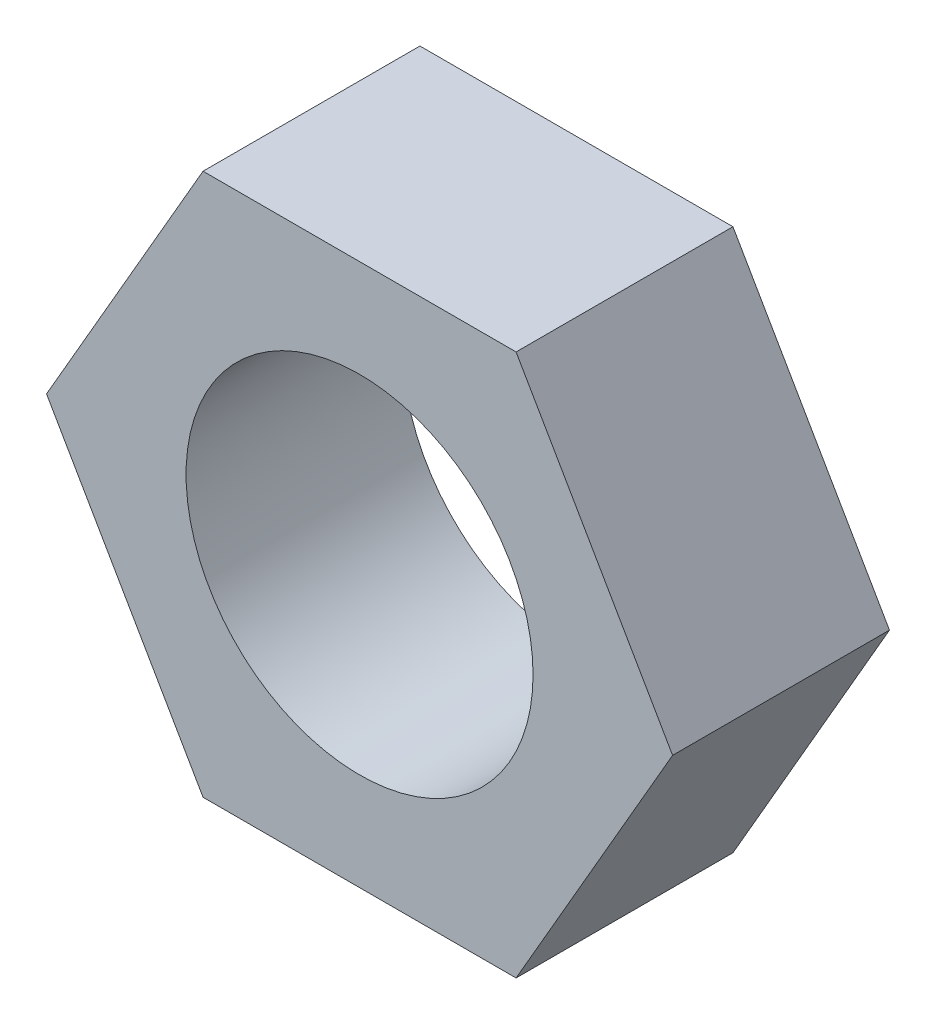
ISO-10303-21;
HEADER;
FILE_DESCRIPTION(('STEP AP214'),'2;1');
FILE_NAME('part.step','',(''),(''),'','','');
FILE_SCHEMA(('AUTOMOTIVE_DESIGN { 1 0 10303 214 1 1 1 1 }'));
ENDSEC;
DATA;
#1=APPLICATION_CONTEXT('core data for automotive mechanical design processes');
#2=APPLICATION_PROTOCOL_DEFINITION('international standard','automotive_design',2000,#1);
#3=PRODUCT_CONTEXT('',#1,'mechanical');
#4=PRODUCT('Part','Part','',(#3));
#5=PRODUCT_RELATED_PRODUCT_CATEGORY('part','',(#4));
#6=PRODUCT_DEFINITION_FORMATION('','',#4);
#7=PRODUCT_DEFINITION_CONTEXT('part definition',#1,'design');
#8=PRODUCT_DEFINITION('design','',#6,#7);
#9=PRODUCT_DEFINITION_SHAPE('','',#8);
#10=(LENGTH_UNIT() NAMED_UNIT(*) SI_UNIT(.MILLI.,.METRE.));
#11=(NAMED_UNIT(*) PLANE_ANGLE_UNIT() SI_UNIT($,.RADIAN.));
#12=(NAMED_UNIT(*) SI_UNIT($,.STERADIAN.) SOLID_ANGLE_UNIT());
#13=UNCERTAINTY_MEASURE_WITH_UNIT(LENGTH_MEASURE(1.E-05),#10,'distance_accuracy_value','');
#14=(GEOMETRIC_REPRESENTATION_CONTEXT(3) GLOBAL_UNCERTAINTY_ASSIGNED_CONTEXT((#13)) GLOBAL_UNIT_ASSIGNED_CONTEXT((#10,
#11,#12)) REPRESENTATION_CONTEXT('',''));
#15=CARTESIAN_POINT('',(0.,0.,0.));
#16=DIRECTION('',(0.,0.,1.));
#17=DIRECTION('',(1.,0.,0.));
#18=AXIS2_PLACEMENT_3D('',#15,#16,#17);
#19=CARTESIAN_POINT('',(7.21687836487047,-12.4999999999999,10.));
#20=DIRECTION('',(-0.866025403784442,0.499999999999995,0.));
#21=DIRECTION('',(-0.499999999999995,-0.866025403784442,0.));
#22=AXIS2_PLACEMENT_3D('',#19,#20,#21);
#23=PLANE('',#22);
#24=DIRECTION('',(0.499999999999995,0.866025403784442,0.));
#25=VECTOR('',#24,1.);
#26=CARTESIAN_POINT('',(7.21687836487047,-12.4999999999999,0.));
#27=LINE('',#26,#25);
#28=CARTESIAN_POINT('',(7.21687836487047,-12.4999999999999,0.));
#29=VERTEX_POINT('',#28);
#30=CARTESIAN_POINT('',(14.4337567297407,0.,0.));
#31=VERTEX_POINT('',#30);
#32=EDGE_CURVE('E122',#29,#31,#27,.T.);
#33=ORIENTED_EDGE('',*,*,#32,.T.);
#34=DIRECTION('',(0.,0.,-1.));
#35=VECTOR('',#34,1.);
#36=CARTESIAN_POINT('',(14.4337567297407,0.,10.));
#37=LINE('',#36,#35);
#38=CARTESIAN_POINT('',(14.4337567297407,0.,10.));
#39=VERTEX_POINT('',#38);
#40=EDGE_CURVE('E11',#39,#31,#37,.T.);
#41=ORIENTED_EDGE('',*,*,#40,.F.);
#42=DIRECTION('',(0.499999999999995,0.866025403784442,0.));
#43=VECTOR('',#42,1.);
#44=CARTESIAN_POINT('',(7.21687836487047,-12.4999999999999,10.));
#45=LINE('',#44,#43);
#46=CARTESIAN_POINT('',(7.21687836487047,-12.4999999999999,10.));
#47=VERTEX_POINT('',#46);
#48=EDGE_CURVE('E133',#47,#39,#45,.T.);
#49=ORIENTED_EDGE('',*,*,#48,.F.);
#50=DIRECTION('',(0.,0.,-1.));
#51=VECTOR('',#50,1.);
#52=CARTESIAN_POINT('',(7.21687836487047,-12.4999999999999,10.));
#53=LINE('',#52,#51);
#54=EDGE_CURVE('E118',#47,#29,#53,.T.);
#55=ORIENTED_EDGE('',*,*,#54,.T.);
#56=EDGE_LOOP('',(#33,#41,#49,#55));
#57=FACE_BOUND('',#56,.T.);
#58=ADVANCED_FACE('F39',(#57),#23,.F.);
#59=CARTESIAN_POINT('',(14.4337567297407,0.,10.));
#60=DIRECTION('',(-0.866025403784438,-0.500000000000001,0.));
#61=DIRECTION('',(0.500000000000001,-0.866025403784438,0.));
#62=AXIS2_PLACEMENT_3D('',#59,#60,#61);
#63=PLANE('',#62);
#64=DIRECTION('',(-0.500000000000001,0.866025403784438,0.));
#65=VECTOR('',#64,1.);
#66=CARTESIAN_POINT('',(14.4337567297407,0.,0.));
#67=LINE('',#66,#65);
#68=CARTESIAN_POINT('',(7.2168783648703,12.5,0.));
#69=VERTEX_POINT('',#68);
#70=EDGE_CURVE('E127',#31,#69,#67,.T.);
#71=ORIENTED_EDGE('',*,*,#70,.T.);
#72=DIRECTION('',(0.,0.,-1.));
#73=VECTOR('',#72,1.);
#74=CARTESIAN_POINT('',(7.2168783648703,12.5,10.));
#75=LINE('',#74,#73);
#76=CARTESIAN_POINT('',(7.2168783648703,12.5,10.));
#77=VERTEX_POINT('',#76);
#78=EDGE_CURVE('E50',#77,#69,#75,.T.);
#79=ORIENTED_EDGE('',*,*,#78,.F.);
#80=DIRECTION('',(-0.500000000000001,0.866025403784438,0.));
#81=VECTOR('',#80,1.);
#82=CARTESIAN_POINT('',(14.4337567297407,0.,10.));
#83=LINE('',#82,#81);
#84=EDGE_CURVE('E95',#39,#77,#83,.T.);
#85=ORIENTED_EDGE('',*,*,#84,.F.);
#86=ORIENTED_EDGE('',*,*,#40,.T.);
#87=EDGE_LOOP('',(#71,#79,#85,#86));
#88=FACE_BOUND('',#87,.T.);
#89=ADVANCED_FACE('F157',(#88),#63,.F.);
#90=CARTESIAN_POINT('',(7.2168783648703,12.5,10.));
#91=DIRECTION('',(0.,-1.,0.));
#92=DIRECTION('',(1.,0.,0.));
#93=AXIS2_PLACEMENT_3D('',#90,#91,#92);
#94=PLANE('',#93);
#95=DIRECTION('',(-1.,0.,0.));
#96=VECTOR('',#95,1.);
#97=CARTESIAN_POINT('',(7.2168783648703,12.5,0.));
#98=LINE('',#97,#96);
#99=CARTESIAN_POINT('',(-7.21687836487038,12.5,0.));
#100=VERTEX_POINT('',#99);
#101=EDGE_CURVE('E129',#69,#100,#98,.T.);
#102=ORIENTED_EDGE('',*,*,#101,.T.);
#103=DIRECTION('',(0.,0.,-1.));
#104=VECTOR('',#103,1.);
#105=CARTESIAN_POINT('',(-7.21687836487038,12.5,10.));
#106=LINE('',#105,#104);
#107=CARTESIAN_POINT('',(-7.21687836487038,12.5,10.));
#108=VERTEX_POINT('',#107);
#109=EDGE_CURVE('E111',#108,#100,#106,.T.);
#110=ORIENTED_EDGE('',*,*,#109,.F.);
#111=DIRECTION('',(-1.,0.,0.));
#112=VECTOR('',#111,1.);
#113=CARTESIAN_POINT('',(7.2168783648703,12.5,10.));
#114=LINE('',#113,#112);
#115=EDGE_CURVE('E104',#77,#108,#114,.T.);
#116=ORIENTED_EDGE('',*,*,#115,.F.);
#117=ORIENTED_EDGE('',*,*,#78,.T.);
#118=EDGE_LOOP('',(#102,#110,#116,#117));
#119=FACE_BOUND('',#118,.T.);
#120=ADVANCED_FACE('F136',(#119),#94,.F.);
#121=CARTESIAN_POINT('',(-7.21687836487038,12.5,10.));
#122=DIRECTION('',(0.866025403784442,-0.499999999999995,0.));
#123=DIRECTION('',(0.499999999999995,0.866025403784442,0.));
#124=AXIS2_PLACEMENT_3D('',#121,#122,#123);
#125=PLANE('',#124);
#126=DIRECTION('',(-0.499999999999995,-0.866025403784441,0.));
#127=VECTOR('',#126,1.);
#128=CARTESIAN_POINT('',(-7.21687836487038,12.5,0.));
#129=LINE('',#128,#127);
#130=CARTESIAN_POINT('',(-14.4337567297407,-1.00790384542582E-13,0.));
#131=VERTEX_POINT('',#130);
#132=EDGE_CURVE('E114',#100,#131,#129,.T.);
#133=ORIENTED_EDGE('',*,*,#132,.T.);
#134=DIRECTION('',(0.,0.,-1.));
#135=VECTOR('',#134,1.);
#136=CARTESIAN_POINT('',(-14.4337567297407,-1.00790384542582E-13,10.));
#137=LINE('',#136,#135);
#138=CARTESIAN_POINT('',(-14.4337567297407,-1.00790384542582E-13,10.));
#139=VERTEX_POINT('',#138);
#140=EDGE_CURVE('E109',#139,#131,#137,.T.);
#141=ORIENTED_EDGE('',*,*,#140,.F.);
#142=DIRECTION('',(-0.499999999999995,-0.866025403784441,0.));
#143=VECTOR('',#142,1.);
#144=CARTESIAN_POINT('',(-7.21687836487038,12.5,10.));
#145=LINE('',#144,#143);
#146=EDGE_CURVE('E97',#108,#139,#145,.T.);
#147=ORIENTED_EDGE('',*,*,#146,.F.);
#148=ORIENTED_EDGE('',*,*,#109,.T.);
#149=EDGE_LOOP('',(#133,#141,#147,#148));
#150=FACE_BOUND('',#149,.T.);
#151=ADVANCED_FACE('F112',(#150),#125,.F.);
#152=CARTESIAN_POINT('',(-14.4337567297407,-1.00790384542582E-13,10.));
#153=DIRECTION('',(0.866025403784435,0.500000000000007,0.));
#154=DIRECTION('',(-0.500000000000007,0.866025403784435,0.));
#155=AXIS2_PLACEMENT_3D('',#152,#153,#154);
#156=PLANE('',#155);
#157=DIRECTION('',(0.500000000000007,-0.866025403784434,0.));
#158=VECTOR('',#157,1.);
#159=CARTESIAN_POINT('',(-14.4337567297407,-1.00790384542582E-13,0.));
#160=LINE('',#159,#158);
#161=CARTESIAN_POINT('',(-7.21687836487021,-12.5000000000001,0.));
#162=VERTEX_POINT('',#161);
#163=EDGE_CURVE('E80',#131,#162,#160,.T.);
#164=ORIENTED_EDGE('',*,*,#163,.T.);
#165=DIRECTION('',(0.,0.,-1.));
#166=VECTOR('',#165,1.);
#167=CARTESIAN_POINT('',(-7.21687836487021,-12.5000000000001,10.));
#168=LINE('',#167,#166);
#169=CARTESIAN_POINT('',(-7.21687836487021,-12.5000000000001,10.));
#170=VERTEX_POINT('',#169);
#171=EDGE_CURVE('E113',#170,#162,#168,.T.);
#172=ORIENTED_EDGE('',*,*,#171,.F.);
#173=DIRECTION('',(0.500000000000007,-0.866025403784434,0.));
#174=VECTOR('',#173,1.);
#175=CARTESIAN_POINT('',(-14.4337567297407,-1.00790384542582E-13,10.));
#176=LINE('',#175,#174);
#177=EDGE_CURVE('E103',#139,#170,#176,.T.);
#178=ORIENTED_EDGE('',*,*,#177,.F.);
#179=ORIENTED_EDGE('',*,*,#140,.T.);
#180=EDGE_LOOP('',(#164,#172,#178,#179));
#181=FACE_BOUND('',#180,.T.);
#182=ADVANCED_FACE('F116',(#181),#156,.F.);
#183=CARTESIAN_POINT('',(-7.21687836487021,-12.5000000000001,10.));
#184=DIRECTION('',(0.,1.,0.));
#185=DIRECTION('',(-1.,0.,0.));
#186=AXIS2_PLACEMENT_3D('',#183,#184,#185);
#187=PLANE('',#186);
#188=DIRECTION('',(1.,0.,0.));
#189=VECTOR('',#188,1.);
#190=CARTESIAN_POINT('',(-7.21687836487021,-12.5000000000001,0.));
#191=LINE('',#190,#189);
#192=EDGE_CURVE('E85',#162,#29,#191,.T.);
#193=ORIENTED_EDGE('',*,*,#192,.T.);
#194=ORIENTED_EDGE('',*,*,#54,.F.);
#195=DIRECTION('',(1.,0.,0.));
#196=VECTOR('',#195,1.);
#197=CARTESIAN_POINT('',(-7.21687836487021,-12.5000000000001,10.));
#198=LINE('',#197,#196);
#199=EDGE_CURVE('E54',#170,#47,#198,.T.);
#200=ORIENTED_EDGE('',*,*,#199,.F.);
#201=ORIENTED_EDGE('',*,*,#171,.T.);
#202=EDGE_LOOP('',(#193,#194,#200,#201));
#203=FACE_BOUND('',#202,.T.);
#204=ADVANCED_FACE('F150',(#203),#187,.F.);
#205=CARTESIAN_POINT('',(0.,0.,10.));
#206=DIRECTION('',(0.,0.,1.));
#207=DIRECTION('',(1.,0.,0.));
#208=AXIS2_PLACEMENT_3D('',#205,#206,#207);
#209=PLANE('',#208);
#210=CARTESIAN_POINT('',(0.,0.,10.));
#211=DIRECTION('',(0.,0.,1.));
#212=DIRECTION('',(1.,0.,0.));
#213=AXIS2_PLACEMENT_3D('',#210,#211,#212);
#214=CIRCLE('',#213,8.);
#215=CARTESIAN_POINT('',(8.,0.,10.));
#216=VERTEX_POINT('',#215);
#217=EDGE_CURVE('E214',#216,#216,#214,.T.);
#218=ORIENTED_EDGE('',*,*,#217,.F.);
#219=EDGE_LOOP('',(#218));
#220=FACE_BOUND('',#219,.T.);
#221=ORIENTED_EDGE('',*,*,#48,.T.);
#222=ORIENTED_EDGE('',*,*,#84,.T.);
#223=ORIENTED_EDGE('',*,*,#115,.T.);
#224=ORIENTED_EDGE('',*,*,#146,.T.);
#225=ORIENTED_EDGE('',*,*,#177,.T.);
#226=ORIENTED_EDGE('',*,*,#199,.T.);
#227=EDGE_LOOP('',(#221,#222,#223,#224,#225,#226));
#228=FACE_BOUND('',#227,.T.);
#229=ADVANCED_FACE('F101',(#220,#228),#209,.T.);
#230=CARTESIAN_POINT('',(0.,0.,0.));
#231=DIRECTION('',(0.,0.,1.));
#232=DIRECTION('',(1.,0.,0.));
#233=AXIS2_PLACEMENT_3D('',#230,#231,#232);
#234=PLANE('',#233);
#235=CARTESIAN_POINT('',(0.,0.,0.));
#236=DIRECTION('',(0.,0.,1.));
#237=DIRECTION('',(1.,0.,0.));
#238=AXIS2_PLACEMENT_3D('',#235,#236,#237);
#239=CIRCLE('',#238,8.);
#240=CARTESIAN_POINT('',(8.,0.,0.));
#241=VERTEX_POINT('',#240);
#242=EDGE_CURVE('E130',#241,#241,#239,.T.);
#243=ORIENTED_EDGE('',*,*,#242,.T.);
#244=EDGE_LOOP('',(#243));
#245=FACE_BOUND('',#244,.T.);
#246=ORIENTED_EDGE('',*,*,#32,.F.);
#247=ORIENTED_EDGE('',*,*,#192,.F.);
#248=ORIENTED_EDGE('',*,*,#163,.F.);
#249=ORIENTED_EDGE('',*,*,#132,.F.);
#250=ORIENTED_EDGE('',*,*,#101,.F.);
#251=ORIENTED_EDGE('',*,*,#70,.F.);
#252=EDGE_LOOP('',(#246,#247,#248,#249,#250,#251));
#253=FACE_BOUND('',#252,.T.);
#254=ADVANCED_FACE('F141',(#245,#253),#234,.F.);
#255=CARTESIAN_POINT('',(0.,0.,0.));
#256=DIRECTION('',(0.,0.,1.));
#257=DIRECTION('',(1.,0.,0.));
#258=AXIS2_PLACEMENT_3D('',#255,#256,#257);
#259=CYLINDRICAL_SURFACE('',#258,8.);
#260=ORIENTED_EDGE('',*,*,#242,.F.);
#261=EDGE_LOOP('',(#260));
#262=FACE_BOUND('',#261,.T.);
#263=ORIENTED_EDGE('',*,*,#217,.T.);
#264=EDGE_LOOP('',(#263));
#265=FACE_BOUND('',#264,.T.);
#266=ADVANCED_FACE('F196',(#262,#265),#259,.F.);
#267=CLOSED_SHELL('',(#58,#89,#120,#151,#182,#204,#229,#254,#266));
#268=MANIFOLD_SOLID_BREP('B2',#267);
#269=ADVANCED_BREP_SHAPE_REPRESENTATION('',(#18,#268),#14);
#270=SHAPE_DEFINITION_REPRESENTATION(#9,#269);
ENDSEC;
END-ISO-10303-21;
